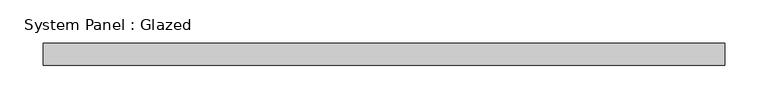
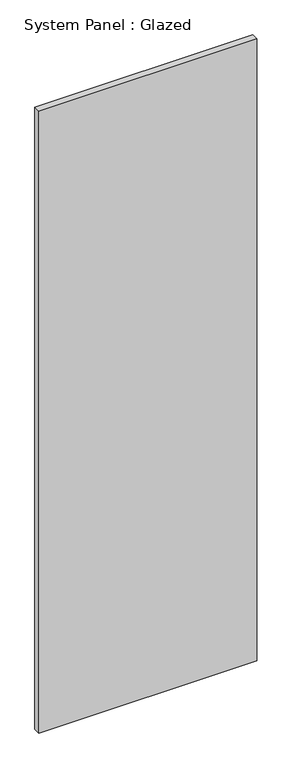
"""IFC4 building model written with IfcOpenShell, lengths in millimetres: plate geometry, System Panel : Glazed."""

from ifc_helpers import new_model, si_unit, origin, origin_with_axes, place, context, project, spatial, polyline, outline, extrude, source, transform, mapped, element, save


def system_panel_glazed_4ec892b8(model_context):
    return source(origin(), model_context, "Body", "SweptSolid", [
        extrude(outline(polyline([(393.7, 19.05), (-393.7, 19.05), (-393.7, 44.45), (393.7, 44.45), (393.7, 19.05)])), origin_with_axes(), (0.0, 0.0, 1.0), 2374.9),
    ])


if __name__ == "__main__":
    model = new_model("IFC4")
    model_context = context("Model", 3, world=origin())
    ifc_project = project(units=[si_unit("LENGTHUNIT", "METRE", prefix="MILLI")], contexts=[model_context])
    site = spatial("IfcSite", under=ifc_project)
    building = spatial("IfcBuilding", under=site)
    placement = place(None, origin())
    system_panel_glazed_shape = system_panel_glazed_4ec892b8(model_context)
    element("IfcPlate", 1, ObjectType="System Panel : Glazed", at=placement, inside=building, context=model_context, shape_type="MappedRepresentation", body=[
        mapped(system_panel_glazed_shape, transform((0.0, 0.0, 0.0), x_axis=(1.0, 0.0, 0.0), y_axis=(0.0, 1.0, 0.0), z_axis=(0.0, 0.0, 1.0))),
    ])
    save(model, "model.ifc")

# Revit data of these elements
# Type "System Panel : Glazed"
#   Construction Type Id = "GSP4R"
#   Analytic Construction = "1/8 in Pilkington single glazing"
#   Visual Light Transmittance = 0.9
#   Solar Heat Gain Coefficient = 0.86
#   Heat Transfer Coefficient (U) = 1.18115 BTU/(h·ft²·°F)
#   Define Thermal Properties by = 1
# Element 1 (IfcPlate, "System Panel : Glazed")
#   Materials on its faces: "Glass"
# Materials
#   "Glass": class "Glass", colour RGB 0 128 192, transparency 0.75, Description = "Soda Lime Glass", Cost = 0
